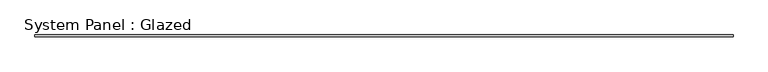
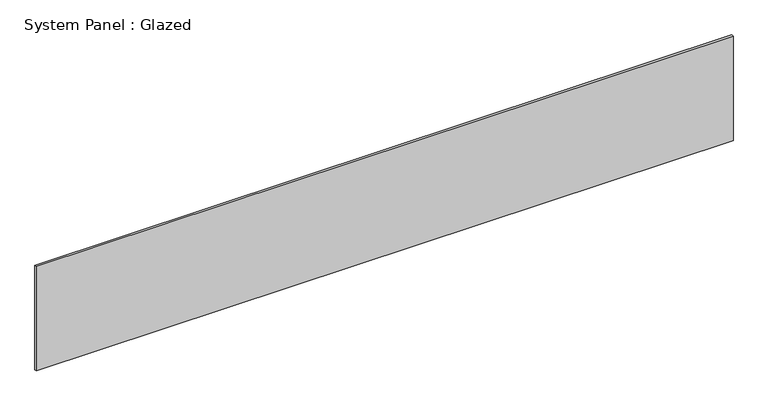
"""IFC4 building model written with IfcOpenShell, lengths in millimetres: plate geometry, System Panel : Glazed."""

from ifc_helpers import new_model, si_unit, origin, origin_with_axes, place, context, project, spatial, polyline, outline, extrude, source, transform, mapped, element, save


def system_panel_glazed_4de2f835(model_context):
    return source(origin(), model_context, "Body", "SweptSolid", [
        extrude(outline(polyline([(4606.925, 19.05), (-4606.925, 19.05), (-4606.925, 44.45), (4606.925, 44.45), (4606.925, 19.05)])), origin_with_axes(), (0.0, 0.0, 1.0), 1460.5),
    ])


if __name__ == "__main__":
    model = new_model("IFC4")
    model_context = context("Model", 3, world=origin())
    ifc_project = project(units=[si_unit("LENGTHUNIT", "METRE", prefix="MILLI")], contexts=[model_context])
    site = spatial("IfcSite", under=ifc_project)
    building = spatial("IfcBuilding", under=site)
    placement = place(None, origin())
    system_panel_glazed_shape = system_panel_glazed_4de2f835(model_context)
    element("IfcPlate", 1, ObjectType="System Panel : Glazed", at=placement, inside=building, context=model_context, shape_type="MappedRepresentation", body=[
        mapped(system_panel_glazed_shape, transform((0.0, 0.0, 0.0), x_axis=(1.0, 0.0, 0.0), y_axis=(0.0, 1.0, 0.0), z_axis=(0.0, 0.0, 1.0))),
    ])
    save(model, "model.ifc")

# Revit data of these elements
# Type "System Panel : Glazed"
#   Construction Type Id = "GSP4R"
#   Analytic Construction = "1/8 in Pilkington single glazing"
#   Visual Light Transmittance = 0.9
#   Solar Heat Gain Coefficient = 0.86
#   Heat Transfer Coefficient (U) = 1.18115 BTU/(h·ft²·°F)
# Element 1 (IfcPlate, "System Panel : Glazed")
#   Materials on its faces: "Glass"
# Materials
#   "Glass": class "Glass", colour RGB 0 128 192, transparency 0.75, Description = "Soda Lime Glass", Cost = 0
